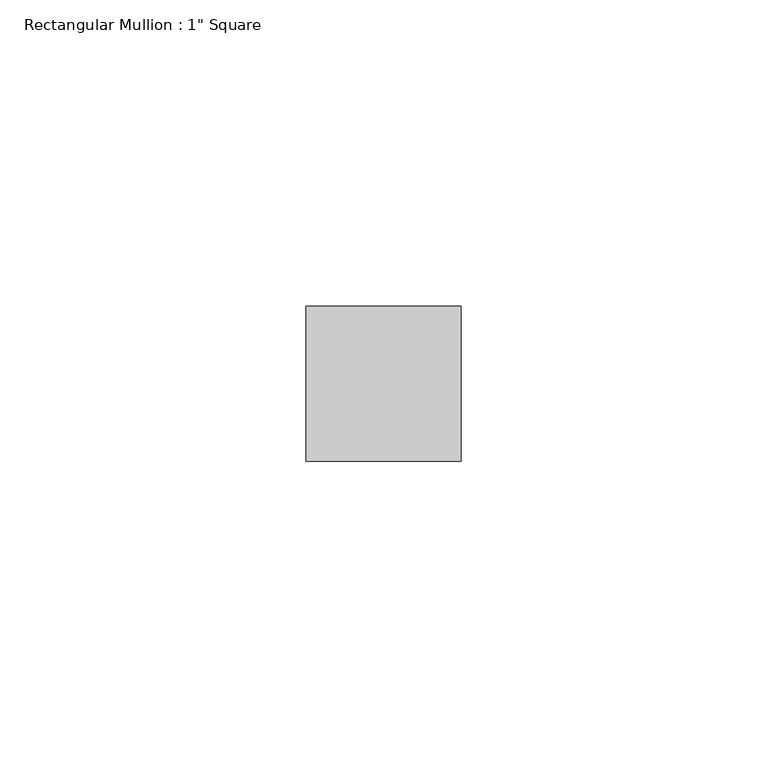
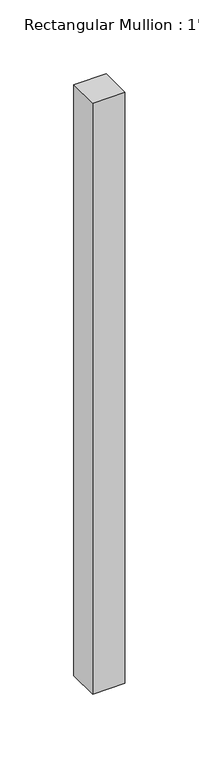
"""IFC4 building model written with IfcOpenShell, lengths in millimetres: member geometry."""

from ifc_helpers import new_model, si_unit, frame, origin, place, context, project, spatial, polyline, outline, extrude, source, transform, mapped, element, save


def member_8b4722c0(model_context):
    return source(origin(), model_context, "Body", "SweptSolid", [
        extrude(outline(polyline([(0.0, 12.7), (0.0, -12.7), (-25.4, -12.7), (-25.4, 12.7), (0.0, 12.7)])), frame((0.0, 0.0, -488.95), z_axis=(0.0, 0.0, 1.0), x_axis=(1.0, 0.0, 0.0)), (0.0, 0.0, 1.0), 488.95),
    ])


if __name__ == "__main__":
    model = new_model("IFC4")
    model_context = context("Model", 3, world=origin())
    ifc_project = project(units=[si_unit("LENGTHUNIT", "METRE", prefix="MILLI")], contexts=[model_context])
    site = spatial("IfcSite", under=ifc_project)
    building = spatial("IfcBuilding", under=site)
    placement = place(None, origin())
    member_shape = member_8b4722c0(model_context)
    element("IfcMember", 1, ObjectType="Rectangular Mullion : 1\" Square", at=placement, inside=building, context=model_context, shape_type="MappedRepresentation", body=[
        mapped(member_shape, transform((0.0, 0.0, 0.0), x_axis=(1.0, 0.0, 0.0), y_axis=(0.0, 1.0, 0.0), z_axis=(0.0, 0.0, 1.0))),
    ])
    save(model, "model.ifc")

# Revit data of these elements
# Type "Rectangular Mullion : 1\" Square"
#   built-in parameter 1007304 = 0.0833333 (stored number, unit not read)
#   built-in parameter 1007301 = 0.0416667 (stored number, unit not read)
#   built-in parameter 1007300 = 0.0416667 (stored number, unit not read)
